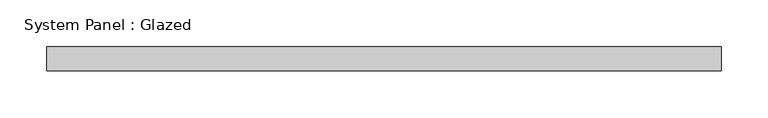
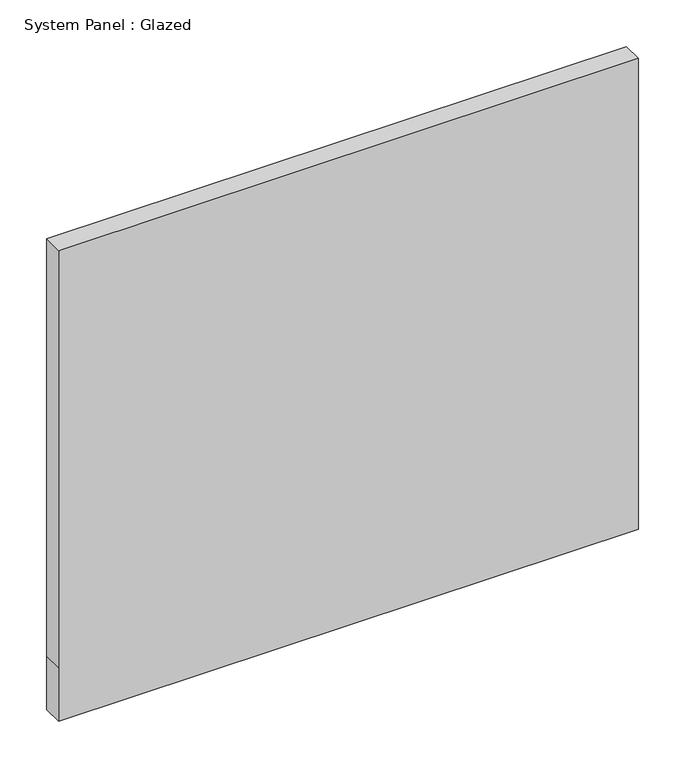
"""IFC4 building model written with IfcOpenShell, lengths in millimetres: plate geometry, System Panel : Glazed."""

from ifc_helpers import new_model, si_unit, frame, origin, place, context, project, spatial, polyline, outline, extrude, source, transform, mapped, element, save


def system_panel_glazed_eced71b2(model_context):
    return source(origin(), model_context, "Body", "SweptSolid", [
        extrude(outline(polyline([(0.0, -358.775), (0.0, 358.775), (69.7832841, 358.775), (615.4829888, 358.775), (615.4829888, -358.775), (69.7832841, -358.775), (0.0, -358.775)])), frame((0.0, 19.05, 0.0), z_axis=(0.0, 1.0, 0.0), x_axis=(0.0, 0.0, 1.0)), (0.0, 0.0, 1.0), 25.4),
    ])


if __name__ == "__main__":
    model = new_model("IFC4")
    model_context = context("Model", 3, world=origin())
    ifc_project = project(units=[si_unit("LENGTHUNIT", "METRE", prefix="MILLI")], contexts=[model_context])
    site = spatial("IfcSite", under=ifc_project)
    building = spatial("IfcBuilding", under=site)
    placement = place(None, origin())
    system_panel_glazed_shape = system_panel_glazed_eced71b2(model_context)
    element("IfcPlate", 1, ObjectType="System Panel : Glazed", at=placement, inside=building, context=model_context, shape_type="MappedRepresentation", body=[
        mapped(system_panel_glazed_shape, transform((0.0, 0.0, 0.0), x_axis=(1.0, 0.0, 0.0), y_axis=(0.0, 1.0, 0.0), z_axis=(0.0, 0.0, 1.0))),
    ])
    save(model, "model.ifc")

# Revit data of these elements
# Type "System Panel : Glazed"
#   Construction Type Id = "GSP4R"
#   Analytic Construction = "1/8 in Pilkington single glazing"
#   Visual Light Transmittance = 0.9
#   Solar Heat Gain Coefficient = 0.86
#   Heat Transfer Coefficient (U) = 1.18115 BTU/(h·ft²·°F)
#   Define Thermal Properties by = 1
# Element 1 (IfcPlate, "System Panel : Glazed")
#   Materials on its faces: "Glass"
# Materials
#   "Glass": class "Glass", colour RGB 0 128 192, transparency 0.75, Description = "Soda Lime Glass", Cost = 0
